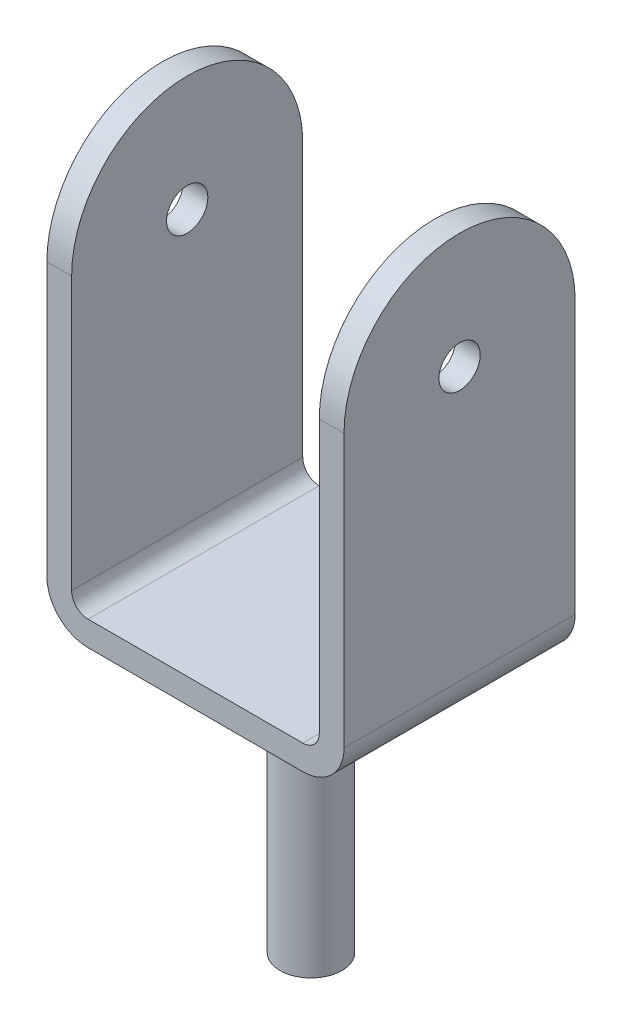
SolidWorks part; units mm, degrees
material "Plain Carbon Steel"
ref_plane "Front Plane" through (0, 0, 0) normal (0, 0, 1) x (1, 0, 0)
ref_plane "Top Plane" through (0, 0, 0) normal (0, 1, 0) x (1, 0, 0)
ref_plane "Right Plane" through (0, 0, 0) normal (1, 0, 0) x (0, 0, -1)
sketch "U-Channel Profile Sketch" plane through (0, 0, 0) normal (0, 0, 1) x (1, 0, 0)
  line L0 (-180, 380) -> (-180, 0)
  line L1 (-180, 0) -> (180, 0)
  line L2 (180, 0) -> (180, 380)
  line L3 (-150, 380) -> (-150, 30)
  line L4 (-150, 30) -> (150, 30)
  line L5 (150, 30) -> (150, 380)
  line L6 (-180, 380) -> (-150, 380)
  line L7 (150, 380) -> (180, 380)
  point P2 (0, 0)
  dimension "D1" = 360
  dimension "D2" = 380
  dimension "D3" = 30
extrude "U-Channel Body" add sketch "U-Channel Profile Sketch" along normal mid plane 280
sketch "Stem Sketch Ø75" plane through (0, 0, 0) normal (0, -1, 0) x (1, 0, 0)
  circle A0 centre (0, 0) radius 37.5
  dimension "D1" = 75
extrude "Stem Ø75" add sketch "Stem Sketch Ø75" along normal blind 325
fillet "Upright Top Rounds R50" radius 50 2 edges at (180, 0, 0) (-180, 0, 0)
ref_plane "Reference Plane" through (-150, 30, -140) normal (0, 0, -1) x (-1, 0, 0)
fillet "Channel Fillets R20" radius 20 2 edges at (-150, 30, 0) (150, 30, 0)
sketch "Side Boss Sketch" plane through (180, 0, 0) normal (1, 0, 0) x (0, 0, -1)
  line L0 (-140, 380) -> (140, 380) construction
  circle A0 centre (0, 380) radius 140
extrude "Side Boss" add sketch "Side Boss Sketch" against normal blind 30
mirror "Side Boss Mirror" about plane through (0, 0, 0) normal (1, 0, 0) of "Side Boss"
sketch "Pin Hole Sketch" plane through (-180, 0, 0) normal (-1, 0, 0) x (0, 0, 1)
  line L0 (140, 0) -> (-140, 0) construction
  circle A0 centre (0, 380) radius 25
  dimension "D1" = 50
  dimension "D2" = 380
extrude "Pin Holes" cut sketch "Pin Hole Sketch" against normal through all
